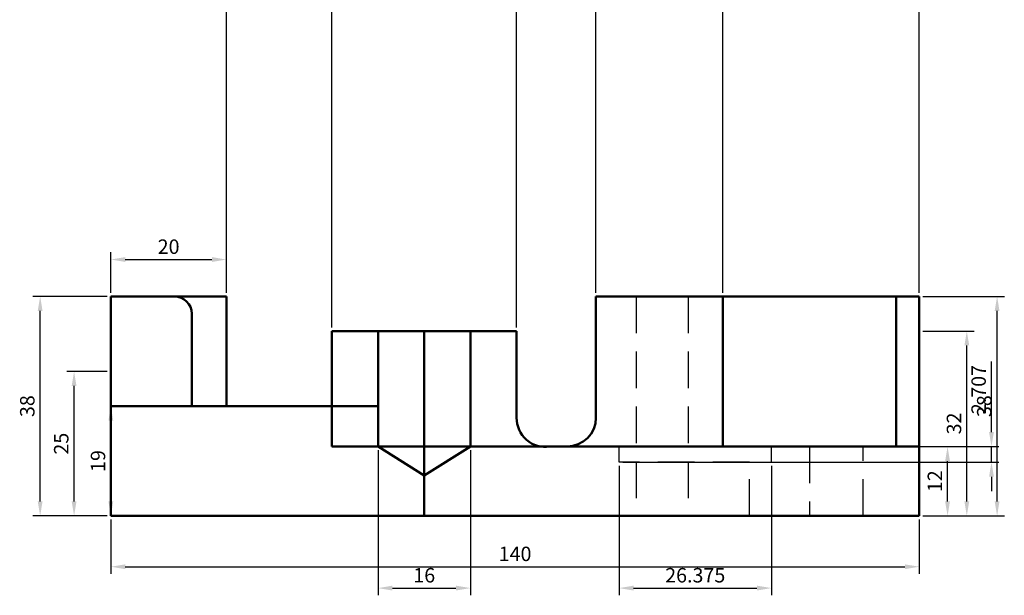
# Model space of a CAD drawing. Units: millimetres. Extents: x 2432 to 2611, y 2100 to 2357.
# Tile 1 of 3: x 2434 to 2605, y 2100 to 2199. Entities that reach past the tile are written whole.
import ezdxf

# ---------------------------------------------------------------- set-up
doc = ezdxf.new("R2010")
doc.units = ezdxf.units.MM
doc.linetypes.add('HIDDEN', pattern=[9.525, 6.35, -3.175])
for name, color, linetype, lineweight in [('M-DIMS', 2, 'Continuous', 25), ('M-HIDN', 8, 'HIDDEN', 25), ('M-OUTL', 7, 'Continuous', 50)]:
    doc.layers.add(name, color=color, linetype=linetype, lineweight=lineweight)
doc.styles.get("Standard").update_dxf_attribs({"font": 'arial.ttf'})
doc.dimstyles.new('ISO-25', dxfattribs={"dimtxt": 2.5, "dimasz": 2.5, "dimexe": 1.25, "dimexo": 0.625, "dimtad": 1, "dimtxsty": 'Standard', "dimcen": 2.5, "dimadec": 0, "dimazin": 0, "dimtfac": 1, "dimtmove": 0, "dimatfit": 3, "dimfxl": 1, "dimarcsym": 0})

# ---------------------------------------------------------------- blocks, each defined once
blk = doc.blocks.new('*D26')
at = {"layer": 'Defpoints', "color": 0, "transparency": 16777216}
for p in [(2437.83, 2151.26), (2450.07, 2151.26), (2450.07, 2113.26)]:
    blk.add_point(p, dxfattribs=at)
at = {"layer": 'M-DIMS', "color": 0, "lineweight": -2, "transparency": 16777216}
for p, q in [((2449.45, 2151.26), (2436.58, 2151.26)), ((2437.83, 2115.76), (2437.83, 2148.76)), ((2449.45, 2113.26), (2436.58, 2113.26))]:
    blk.add_line(p, q, dxfattribs=at)
at = {"layer": 'M-DIMS', "color": 0, "transparency": 16777216}
for points in [[(2437.41, 2148.76), (2438.24, 2148.76), (2437.83, 2151.26)], [(2437.41, 2115.76), (2438.24, 2115.76), (2437.83, 2113.26)]]:
    blk.add_solid(points, dxfattribs=at)
at = {"layer": 'M-DIMS', "color": 0, "transparency": 16777216, "insert": (2435.92, 2132.26), "char_height": 2.5, "attachment_point": 5, "rotation": 90}
blk.add_mtext('38', dxfattribs=at)
blk = doc.blocks.new('*D27')
at = {"layer": 'Defpoints', "color": 0, "transparency": 16777216}
for p in [(2443.7, 2138.26), (2450.07, 2138.26), (2450.07, 2113.26)]:
    blk.add_point(p, dxfattribs=at)
at = {"layer": 'M-DIMS', "color": 0, "lineweight": -2, "transparency": 16777216}
for p, q in [((2449.45, 2138.26), (2442.45, 2138.26)), ((2443.7, 2115.76), (2443.7, 2135.76)), ((2449.45, 2113.26), (2442.45, 2113.26))]:
    blk.add_line(p, q, dxfattribs=at)
at = {"layer": 'M-DIMS', "color": 0, "transparency": 16777216}
for points in [[(2443.29, 2135.76), (2444.12, 2135.76), (2443.7, 2138.26)], [(2443.29, 2115.76), (2444.12, 2115.76), (2443.7, 2113.26)]]:
    blk.add_solid(points, dxfattribs=at)
at = {"layer": 'M-DIMS', "color": 0, "transparency": 16777216, "insert": (2441.8, 2125.76), "char_height": 2.5, "attachment_point": 5, "rotation": 90}
blk.add_mtext('25', dxfattribs=at)
blk = doc.blocks.new('*D28')
at = {"layer": 'Defpoints', "color": 0, "transparency": 16777216}
for p in [(2450.07, 2132.26), (2450.07, 2132.26), (2450.07, 2113.26)]:
    blk.add_point(p, dxfattribs=at)
at = {"layer": 'M-DIMS', "color": 0, "lineweight": -2, "transparency": 16777216}
for p, q in [((2450.7, 2132.26), (2451.32, 2132.26)), ((2450.07, 2115.76), (2450.07, 2129.76)), ((2450.7, 2113.26), (2451.32, 2113.26))]:
    blk.add_line(p, q, dxfattribs=at)
at = {"layer": 'M-DIMS', "color": 0, "transparency": 16777216}
for points in [[(2449.66, 2129.76), (2450.49, 2129.76), (2450.07, 2132.26)], [(2449.66, 2115.76), (2450.49, 2115.76), (2450.07, 2113.26)]]:
    blk.add_solid(points, dxfattribs=at)
at = {"layer": 'M-DIMS', "color": 0, "transparency": 16777216, "insert": (2448.17, 2122.76), "char_height": 2.5, "attachment_point": 5, "rotation": 90}
blk.add_mtext('19', dxfattribs=at)
blk = doc.blocks.new('*D29')
at = {"layer": 'Defpoints', "color": 0, "transparency": 16777216}
for p in [(2590.07, 2125.26), (2594.97, 2125.26), (2590.07, 2113.26)]:
    blk.add_point(p, dxfattribs=at)
at = {"layer": 'M-DIMS', "color": 0, "lineweight": -2, "transparency": 16777216}
for p, q in [((2590.7, 2125.26), (2596.22, 2125.26)), ((2594.97, 2115.76), (2594.97, 2122.76)), ((2590.7, 2113.26), (2596.22, 2113.26))]:
    blk.add_line(p, q, dxfattribs=at)
at = {"layer": 'M-DIMS', "color": 0, "transparency": 16777216}
for points in [[(2594.55, 2122.76), (2595.38, 2122.76), (2594.97, 2125.26)], [(2594.55, 2115.76), (2595.38, 2115.76), (2594.97, 2113.26)]]:
    blk.add_solid(points, dxfattribs=at)
at = {"layer": 'M-DIMS', "color": 0, "transparency": 16777216, "insert": (2593.09, 2119.26), "char_height": 2.5, "attachment_point": 5, "rotation": 90}
blk.add_mtext('12', dxfattribs=at)
blk = doc.blocks.new('*D30')
at = {"layer": 'Defpoints', "color": 0, "transparency": 16777216}
for p in [(2590.07, 2145.26), (2598.3, 2145.26), (2590.07, 2113.26)]:
    blk.add_point(p, dxfattribs=at)
at = {"layer": 'M-DIMS', "color": 0, "lineweight": -2, "transparency": 16777216}
for p, q in [((2590.7, 2145.26), (2599.55, 2145.26)), ((2598.3, 2115.76), (2598.3, 2142.76)), ((2590.7, 2113.26), (2599.55, 2113.26))]:
    blk.add_line(p, q, dxfattribs=at)
at = {"layer": 'M-DIMS', "color": 0, "transparency": 16777216}
for points in [[(2597.89, 2142.76), (2598.72, 2142.76), (2598.3, 2145.26)], [(2597.89, 2115.76), (2598.72, 2115.76), (2598.3, 2113.26)]]:
    blk.add_solid(points, dxfattribs=at)
at = {"layer": 'M-DIMS', "color": 0, "transparency": 16777216, "insert": (2596.4, 2129.26), "char_height": 2.5, "attachment_point": 5, "rotation": 90}
blk.add_mtext('32', dxfattribs=at)
blk = doc.blocks.new('*D31')
at = {"layer": 'Defpoints', "color": 0, "transparency": 16777216}
for p in [(2590.07, 2151.26), (2603.55, 2151.26), (2590.07, 2113.26)]:
    blk.add_point(p, dxfattribs=at)
at = {"layer": 'M-DIMS', "color": 0, "lineweight": -2, "transparency": 16777216}
for p, q in [((2590.7, 2151.26), (2604.8, 2151.26)), ((2603.55, 2115.76), (2603.55, 2148.76)), ((2590.7, 2113.26), (2604.8, 2113.26))]:
    blk.add_line(p, q, dxfattribs=at)
at = {"layer": 'M-DIMS', "color": 0, "transparency": 16777216}
for points in [[(2603.13, 2148.76), (2603.96, 2148.76), (2603.55, 2151.26)], [(2603.13, 2115.76), (2603.96, 2115.76), (2603.55, 2113.26)]]:
    blk.add_solid(points, dxfattribs=at)
at = {"layer": 'M-DIMS', "color": 0, "transparency": 16777216, "insert": (2601.64, 2132.26), "char_height": 2.5, "attachment_point": 5, "rotation": 90}
blk.add_mtext('38', dxfattribs=at)
blk = doc.blocks.new('*D32')
at = {"layer": 'Defpoints', "color": 0, "transparency": 16777216}
for p in [(2450.07, 2113.26), (2590.07, 2113.26), (2590.07, 2104.46)]:
    blk.add_point(p, dxfattribs=at)
at = {"layer": 'M-DIMS', "color": 0, "lineweight": -2, "transparency": 16777216}
for p, q in [((2450.07, 2112.64), (2450.07, 2103.21)), ((2590.07, 2112.64), (2590.07, 2103.21)), ((2452.57, 2104.46), (2587.57, 2104.46))]:
    blk.add_line(p, q, dxfattribs=at)
at = {"layer": 'M-DIMS', "color": 0, "transparency": 16777216}
for points in [[(2452.57, 2104.87), (2452.57, 2104.04), (2450.07, 2104.46)], [(2587.57, 2104.87), (2587.57, 2104.04), (2590.07, 2104.46)]]:
    blk.add_solid(points, dxfattribs=at)
at = {"layer": 'M-DIMS', "color": 0, "transparency": 16777216, "insert": (2520.07, 2106.36), "char_height": 2.5, "attachment_point": 5}
blk.add_mtext('140', dxfattribs=at)
blk = doc.blocks.new('*D33')
at = {"layer": 'Defpoints', "color": 0, "transparency": 16777216}
for p in [(2470.07, 2157.64), (2450.07, 2151.26), (2470.07, 2151.26)]:
    blk.add_point(p, dxfattribs=at)
at = {"layer": 'M-DIMS', "color": 0, "lineweight": -2, "transparency": 16777216}
for p, q in [((2450.07, 2151.89), (2450.07, 2158.89)), ((2470.07, 2151.89), (2470.07, 2158.89)), ((2452.57, 2157.64), (2467.57, 2157.64))]:
    blk.add_line(p, q, dxfattribs=at)
at = {"layer": 'M-DIMS', "color": 0, "transparency": 16777216}
for points in [[(2452.57, 2158.06), (2452.57, 2157.22), (2450.07, 2157.64)], [(2467.57, 2158.06), (2467.57, 2157.22), (2470.07, 2157.64)]]:
    blk.add_solid(points, dxfattribs=at)
at = {"layer": 'M-DIMS', "color": 0, "transparency": 16777216, "insert": (2460.07, 2159.54), "char_height": 2.5, "attachment_point": 5}
blk.add_mtext('20', dxfattribs=at)
blk = doc.blocks.new('*D43')
at = {"layer": 'Defpoints', "color": 0, "transparency": 16777216}
for p in [(2488.34, 2353.19), (2470.07, 2151.26), (2488.34, 2145.26)]:
    blk.add_point(p, dxfattribs=at)
at = {"layer": 'M-DIMS', "color": 0, "lineweight": -2, "transparency": 16777216}
for p, q in [((2470.07, 2151.89), (2470.07, 2354.44)), ((2472.57, 2353.19), (2485.84, 2353.19)), ((2488.34, 2145.89), (2488.34, 2354.44))]:
    blk.add_line(p, q, dxfattribs=at)
at = {"layer": 'M-DIMS', "color": 0, "transparency": 16777216}
for points in [[(2472.57, 2353.6), (2472.57, 2352.77), (2470.07, 2353.19)], [(2485.84, 2353.6), (2485.84, 2352.77), (2488.34, 2353.19)]]:
    blk.add_solid(points, dxfattribs=at)
at = {"layer": 'M-DIMS', "color": 0, "transparency": 16777216, "insert": (2479.21, 2355.09), "char_height": 2.5, "attachment_point": 5}
blk.add_mtext('18.265', dxfattribs=at)
blk = doc.blocks.new('*D44')
at = {"layer": 'Defpoints', "color": 0, "transparency": 16777216}
for p in [(2520.34, 2353.19), (2488.34, 2145.26), (2520.34, 2145.26)]:
    blk.add_point(p, dxfattribs=at)
at = {"layer": 'M-DIMS', "color": 0, "lineweight": -2, "transparency": 16777216}
for p, q in [((2488.34, 2145.89), (2488.34, 2354.44)), ((2490.84, 2353.19), (2517.84, 2353.19)), ((2520.34, 2145.89), (2520.34, 2354.44))]:
    blk.add_line(p, q, dxfattribs=at)
at = {"layer": 'M-DIMS', "color": 0, "transparency": 16777216}
for points in [[(2490.84, 2353.6), (2490.84, 2352.77), (2488.34, 2353.19)], [(2517.84, 2353.6), (2517.84, 2352.77), (2520.34, 2353.19)]]:
    blk.add_solid(points, dxfattribs=at)
at = {"layer": 'M-DIMS', "color": 0, "transparency": 16777216, "insert": (2504.34, 2355.09), "char_height": 2.5, "attachment_point": 5}
blk.add_mtext('32', dxfattribs=at)
blk = doc.blocks.new('*D45')
at = {"layer": 'Defpoints', "color": 0, "transparency": 16777216}
for p in [(2534.07, 2353.19), (2534.07, 2151.26), (2520.34, 2145.26)]:
    blk.add_point(p, dxfattribs=at)
at = {"layer": 'M-DIMS', "color": 0, "lineweight": -2, "transparency": 16777216}
for p, q in [((2520.34, 2145.89), (2520.34, 2354.44)), ((2522.84, 2353.19), (2531.57, 2353.19)), ((2534.07, 2151.89), (2534.07, 2354.44))]:
    blk.add_line(p, q, dxfattribs=at)
at = {"layer": 'M-DIMS', "color": 0, "transparency": 16777216}
for points in [[(2522.84, 2353.6), (2522.84, 2352.77), (2520.34, 2353.19)], [(2531.57, 2353.6), (2531.57, 2352.77), (2534.07, 2353.19)]]:
    blk.add_solid(points, dxfattribs=at)
at = {"layer": 'M-DIMS', "color": 0, "transparency": 16777216, "insert": (2527.21, 2355.09), "char_height": 2.5, "attachment_point": 5}
blk.add_mtext('13.735', dxfattribs=at)
blk = doc.blocks.new('*D46')
at = {"layer": 'Defpoints', "color": 0, "transparency": 16777216}
for p in [(2556.07, 2353.19), (2534.07, 2151.26), (2556.07, 2151.26)]:
    blk.add_point(p, dxfattribs=at)
at = {"layer": 'M-DIMS', "color": 0, "lineweight": -2, "transparency": 16777216}
for p, q in [((2534.07, 2151.89), (2534.07, 2354.44)), ((2536.57, 2353.19), (2553.57, 2353.19)), ((2556.07, 2151.89), (2556.07, 2354.44))]:
    blk.add_line(p, q, dxfattribs=at)
at = {"layer": 'M-DIMS', "color": 0, "transparency": 16777216}
for points in [[(2536.57, 2353.6), (2536.57, 2352.77), (2534.07, 2353.19)], [(2553.57, 2353.6), (2553.57, 2352.77), (2556.07, 2353.19)]]:
    blk.add_solid(points, dxfattribs=at)
at = {"layer": 'M-DIMS', "color": 0, "transparency": 16777216, "insert": (2545.07, 2355.07), "char_height": 2.5, "attachment_point": 5}
blk.add_mtext('22', dxfattribs=at)
blk = doc.blocks.new('*D47')
at = {"layer": 'Defpoints', "color": 0, "transparency": 16777216}
for p in [(2590.07, 2353.19), (2556.07, 2151.26), (2590.07, 2151.26)]:
    blk.add_point(p, dxfattribs=at)
at = {"layer": 'M-DIMS', "color": 0, "lineweight": -2, "transparency": 16777216}
for p, q in [((2556.07, 2151.89), (2556.07, 2354.44)), ((2558.57, 2353.19), (2587.57, 2353.19)), ((2590.07, 2151.89), (2590.07, 2354.44))]:
    blk.add_line(p, q, dxfattribs=at)
at = {"layer": 'M-DIMS', "color": 0, "transparency": 16777216}
for points in [[(2558.57, 2353.6), (2558.57, 2352.77), (2556.07, 2353.19)], [(2587.57, 2353.6), (2587.57, 2352.77), (2590.07, 2353.19)]]:
    blk.add_solid(points, dxfattribs=at)
at = {"layer": 'M-DIMS', "color": 0, "transparency": 16777216, "insert": (2573.07, 2355.09), "char_height": 2.5, "attachment_point": 5}
blk.add_mtext('34', dxfattribs=at)
blk = doc.blocks.new('*D48')
at = {"layer": 'Defpoints', "color": 0, "transparency": 16777216}
for p in [(2496.34, 2125.26), (2512.34, 2125.26), (2512.34, 2100.76)]:
    blk.add_point(p, dxfattribs=at)
at = {"layer": 'M-DIMS', "color": 0, "lineweight": -2, "transparency": 16777216}
for p, q in [((2496.34, 2124.64), (2496.34, 2099.51)), ((2512.34, 2124.64), (2512.34, 2099.51)), ((2498.84, 2100.76), (2509.84, 2100.76))]:
    blk.add_line(p, q, dxfattribs=at)
at = {"layer": 'M-DIMS', "color": 0, "transparency": 16777216}
for points in [[(2498.84, 2101.18), (2498.84, 2100.34), (2496.34, 2100.76)], [(2509.84, 2101.18), (2509.84, 2100.34), (2512.34, 2100.76)]]:
    blk.add_solid(points, dxfattribs=at)
at = {"layer": 'M-DIMS', "color": 0, "transparency": 16777216, "insert": (2504.34, 2102.66), "char_height": 2.5, "attachment_point": 5}
blk.add_mtext('16', dxfattribs=at)
blk = doc.blocks.new('*D49')
at = {"layer": 'Defpoints', "color": 0, "transparency": 16777216}
for p in [(2538.08, 2125.26), (2602.57, 2125.26), (2538.08, 2122.55)]:
    blk.add_point(p, dxfattribs=at)
at = {"layer": 'M-DIMS', "color": 0, "lineweight": -2, "transparency": 16777216}
for p, q in [((2602.57, 2127.76), (2602.57, 2139.99)), ((2538.71, 2125.26), (2603.82, 2125.26)), ((2602.57, 2122.55), (2602.57, 2125.26)), ((2538.71, 2122.55), (2603.82, 2122.55)), ((2602.57, 2120.05), (2602.57, 2117.55))]:
    blk.add_line(p, q, dxfattribs=at)
at = {"layer": 'M-DIMS', "color": 0, "transparency": 16777216}
for points in [[(2602.16, 2127.76), (2602.99, 2127.76), (2602.57, 2125.26)], [(2602.16, 2120.05), (2602.99, 2120.05), (2602.57, 2122.55)]]:
    blk.add_solid(points, dxfattribs=at)
at = {"layer": 'M-DIMS', "color": 0, "transparency": 16777216, "insert": (2600.67, 2135.13), "char_height": 2.5, "attachment_point": 5, "rotation": 90}
blk.add_mtext('2.707', dxfattribs=at)
blk = doc.blocks.new('*D50')
at = {"layer": 'Defpoints', "color": 0, "transparency": 16777216}
for p in [(2538.08, 2122.55), (2564.46, 2122.55), (2564.46, 2100.76)]:
    blk.add_point(p, dxfattribs=at)
at = {"layer": 'M-DIMS', "color": 0, "lineweight": -2, "transparency": 16777216}
for p, q in [((2538.08, 2121.93), (2538.08, 2099.51)), ((2564.46, 2121.93), (2564.46, 2099.51)), ((2540.58, 2100.76), (2561.96, 2100.76))]:
    blk.add_line(p, q, dxfattribs=at)
at = {"layer": 'M-DIMS', "color": 0, "transparency": 16777216}
for points in [[(2540.58, 2101.18), (2540.58, 2100.34), (2538.08, 2100.76)], [(2561.96, 2101.18), (2561.96, 2100.34), (2564.46, 2100.76)]]:
    blk.add_solid(points, dxfattribs=at)
at = {"layer": 'M-DIMS', "color": 0, "transparency": 16777216, "insert": (2551.27, 2102.66), "char_height": 2.5, "attachment_point": 5}
blk.add_mtext('26.375', dxfattribs=at)

msp = doc.modelspace()

# ---------------------------------------------------------------- linework, layer by layer
at = {"layer": 'M-HIDN'}
for p, q in [((2541.0681, 2151.2616), (2541.0681, 2113.2616)), ((2550.0745, 2151.2616), (2550.0745, 2113.2616)), ((2538.0834, 2122.5547), (2538.0834, 2125.2616)), ((2564.4587, 2122.5547), (2564.4587, 2125.2616)), ((2580.3475, 2125.2616), (2571.0745, 2125.2616)), ((2571.0745, 2125.2616), (2571.0745, 2113.2616)), ((2580.3475, 2113.2616), (2580.3475, 2125.2616)), ((2560.6454, 2122.5547), (2538.0834, 2122.5547)), ((2560.6454, 2113.2616), (2560.6454, 2122.5547)), ((2560.6454, 2122.5547), (2564.4587, 2122.5547)), ((2571.0745, 2113.2616), (2560.6454, 2113.2616))]:
    msp.add_line(p, q, dxfattribs=at)
at = {"layer": 'M-OUTL'}
for p, q in [((2450.0745, 2151.2616), (2470.0745, 2151.2616)), ((2450.0745, 2113.2616), (2450.0745, 2151.2616)), ((2450.0745, 2151.2616), (2470.0745, 2151.2616)), ((2450.0745, 2151.2616), (2464.0745, 2151.2616)), ((2464.0745, 2151.2616), (2461.0745, 2151.2616)), ((2470.0745, 2151.2616), (2470.0745, 2132.2616)), ((2534.0745, 2130.2616), (2534.0745, 2151.2616)), ((2534.0745, 2151.2616), (2544.0745, 2151.2616)), ((2534.0745, 2151.2616), (2590.0745, 2151.2616)), ((2544.0745, 2151.2616), (2556.0745, 2151.2616)), ((2556.0745, 2151.2616), (2556.0745, 2125.2616)), ((2590.0745, 2151.2616), (2586.0745, 2151.2616)), ((2586.0745, 2151.2616), (2586.0745, 2125.2616)), ((2590.0745, 2151.2616), (2590.0745, 2113.2616)), ((2464.0745, 2148.2616), (2464.0745, 2132.2616)), ((2488.3395, 2125.2616), (2488.3395, 2145.2616)), ((2488.3395, 2145.2616), (2494.0745, 2145.2616)), ((2494.0745, 2145.2616), (2520.3395, 2145.2616)), ((2496.3395, 2125.2616), (2496.3395, 2145.2616)), ((2504.3395, 2145.2616), (2504.3395, 2113.2616)), ((2504.3395, 2145.2616), (2512.3395, 2145.2616)), ((2504.3395, 2145.2616), (2520.3395, 2145.2616)), ((2512.3395, 2145.2616), (2512.3395, 2125.2616)), ((2520.3395, 2145.2616), (2520.3395, 2130.1528)), ((2450.0745, 2113.2616), (2450.0745, 2132.2616)), ((2450.0745, 2132.2616), (2485.0745, 2132.2616)), ((2470.0745, 2132.2616), (2488.3395, 2132.2616)), ((2485.0745, 2132.2616), (2488.3395, 2132.2616)), ((2488.3395, 2132.2616), (2496.3395, 2132.2616)), ((2496.3395, 2132.2616), (2496.3395, 2125.2616)), ((2520.3395, 2130.1528), (2520.3395, 2130.2616)), ((2520.3395, 2125.2616), (2488.3395, 2125.2616)), ((2504.3395, 2125.2616), (2494.0745, 2125.2616)), ((2512.3395, 2125.2616), (2496.3395, 2125.2616)), ((2496.3395, 2125.2616), (2504.3395, 2120.2377)), ((2504.3395, 2113.2616), (2504.3395, 2125.2616)), ((2504.3395, 2125.2616), (2590.0745, 2125.2616)), ((2504.3395, 2120.2377), (2512.3395, 2125.2616)), ((2520.3395, 2125.2616), (2525.3395, 2125.2616)), ((2526.0745, 2125.2616), (2534.0745, 2125.2616)), ((2534.0745, 2125.2616), (2529.0745, 2125.2616)), ((2556.0745, 2125.2616), (2586.0745, 2125.2616)), ((2590.0745, 2113.2616), (2450.0745, 2113.2616))]:
    msp.add_line(p, q, dxfattribs=at)
for centre, radius, start, end in [((2461.0745, 2148.2616), 3, 0, 90), ((2525.3392, 2130.2072), 5, 179.377051, 278.45654), ((2529.0745, 2130.2616), 5, 270, 0)]:
    msp.add_arc(centre, radius, start, end, dxfattribs=at)

# ---------------------------------------------------------------- dimensions: what is measured, and where the dimension line sits
at = {"layer": 'M-DIMS'}
for base, p1, p2, override, picture, middle in [((2488.3395, 2353.1874), (2470.0745, 2151.2616), (2488.3395, 2145.2616), {"dimdec": 3, "dimlfac": 1, "dimrnd": 0, "dimzin": 0, "dimdsep": 46, "dimlunit": 2}, '*D43', (2479.207, 2355.0889)), ((2520.3395, 2353.1874), (2488.3395, 2145.2616), (2520.3395, 2145.2616), {"dimdec": 0, "dimlfac": 1, "dimrnd": 0, "dimzin": 0, "dimdsep": 46, "dimlunit": 2}, '*D44', (2504.3395, 2355.0897)), ((2534.0745, 2353.1874), (2520.3395, 2145.2616), (2534.0745, 2151.2616), {"dimdec": 3, "dimlfac": 1, "dimrnd": 0, "dimzin": 0, "dimdsep": 46, "dimlunit": 2}, '*D45', (2527.207, 2355.0897)), ((2556.0745, 2353.1874), (2534.0745, 2151.2616), (2556.0745, 2151.2616), {"dimdec": 0, "dimlfac": 1, "dimrnd": 0, "dimzin": 0, "dimdsep": 46, "dimlunit": 2}, '*D46', (2545.0745, 2355.0676)), ((2590.0745, 2353.1874), (2556.0745, 2151.2616), (2590.0745, 2151.2616), {"dimdec": 0, "dimlfac": 1, "dimrnd": 0, "dimzin": 0, "dimdsep": 46, "dimlunit": 2}, '*D47', (2573.0745, 2355.0897)), ((2470.0745, 2157.6388), (2450.0745, 2151.2616), (2470.0745, 2151.2616), {"dimclrd": 0, "dimclre": 0, "dimclrt": 0}, '*D33', (2460.0745, 2159.5402)), ((2512.3395, 2100.7616), (2496.3395, 2125.2616), (2512.3395, 2125.2616), {"dimdec": 0, "dimlfac": 1, "dimrnd": 0, "dimzin": 0, "dimdsep": 46, "dimlunit": 2}, '*D48', (2504.3395, 2102.663)), ((2564.4587, 2100.7616), (2538.0834, 2122.5547), (2564.4587, 2122.5547), {"dimdec": 3, "dimlfac": 1, "dimrnd": 0, "dimzin": 0, "dimdsep": 46, "dimlunit": 2}, '*D50', (2551.2711, 2102.6639)), ((2590.0745, 2104.457), (2450.0745, 2113.2616), (2590.0745, 2113.2616), {"dimclrd": 0, "dimclre": 0, "dimclrt": 0}, '*D32', (2520.0745, 2106.3585))]:
    dim = msp.add_linear_dim(base=base, p1=p1, p2=p2, dimstyle='ISO-25', override=override, dxfattribs=at)
    dim.commit()
    dim.dimension.update_dxf_attribs({"geometry": picture, "text_midpoint": middle})
for base, p1, p2, override, picture, middle in [((2437.8251, 2151.2616), (2450.0745, 2113.2616), (2450.0745, 2151.2616), {"dimclrd": 0, "dimclre": 0, "dimclrt": 0}, '*D26', (2435.9228, 2132.2616)), ((2603.5452, 2151.2616), (2590.0745, 2113.2616), (2590.0745, 2151.2616), {"dimclrd": 0, "dimclre": 0, "dimclrt": 0}, '*D31', (2601.6429, 2132.2616)), ((2598.3019, 2145.2616), (2590.0745, 2113.2616), (2590.0745, 2145.2616), {"dimclrd": 0, "dimclre": 0, "dimclrt": 0}, '*D30', (2596.3996, 2129.2616)), ((2602.5745, 2125.2616), (2538.0834, 2122.5547), (2538.0834, 2125.2616), {"dimdec": 3, "dimlfac": 1, "dimrnd": 0, "dimzin": 0, "dimdsep": 46, "dimlunit": 2}, '*D49', (2600.6731, 2135.126)), ((2443.7039, 2138.2616), (2450.0745, 2113.2616), (2450.0745, 2138.2616), {"dimclrd": 0, "dimclre": 0, "dimclrt": 0}, '*D27', (2441.8025, 2125.7616)), ((2450.0745, 2132.2616), (2450.0745, 2113.2616), (2450.0745, 2132.2616), {"dimclrd": 0, "dimclre": 0, "dimclrt": 0}, '*D28', (2448.1731, 2122.7616)), ((2594.9652, 2125.2616), (2590.0745, 2113.2616), (2590.0745, 2125.2616), {"dimclrd": 0, "dimclre": 0, "dimclrt": 0}, '*D29', (2593.0851, 2119.2616))]:
    dim = msp.add_linear_dim(base=base, p1=p1, p2=p2, angle=90, dimstyle='ISO-25', override=override, dxfattribs=at)
    dim.commit()
    dim.dimension.update_dxf_attribs({"geometry": picture, "text_midpoint": middle})

doc.saveas('drawing.dxf')
